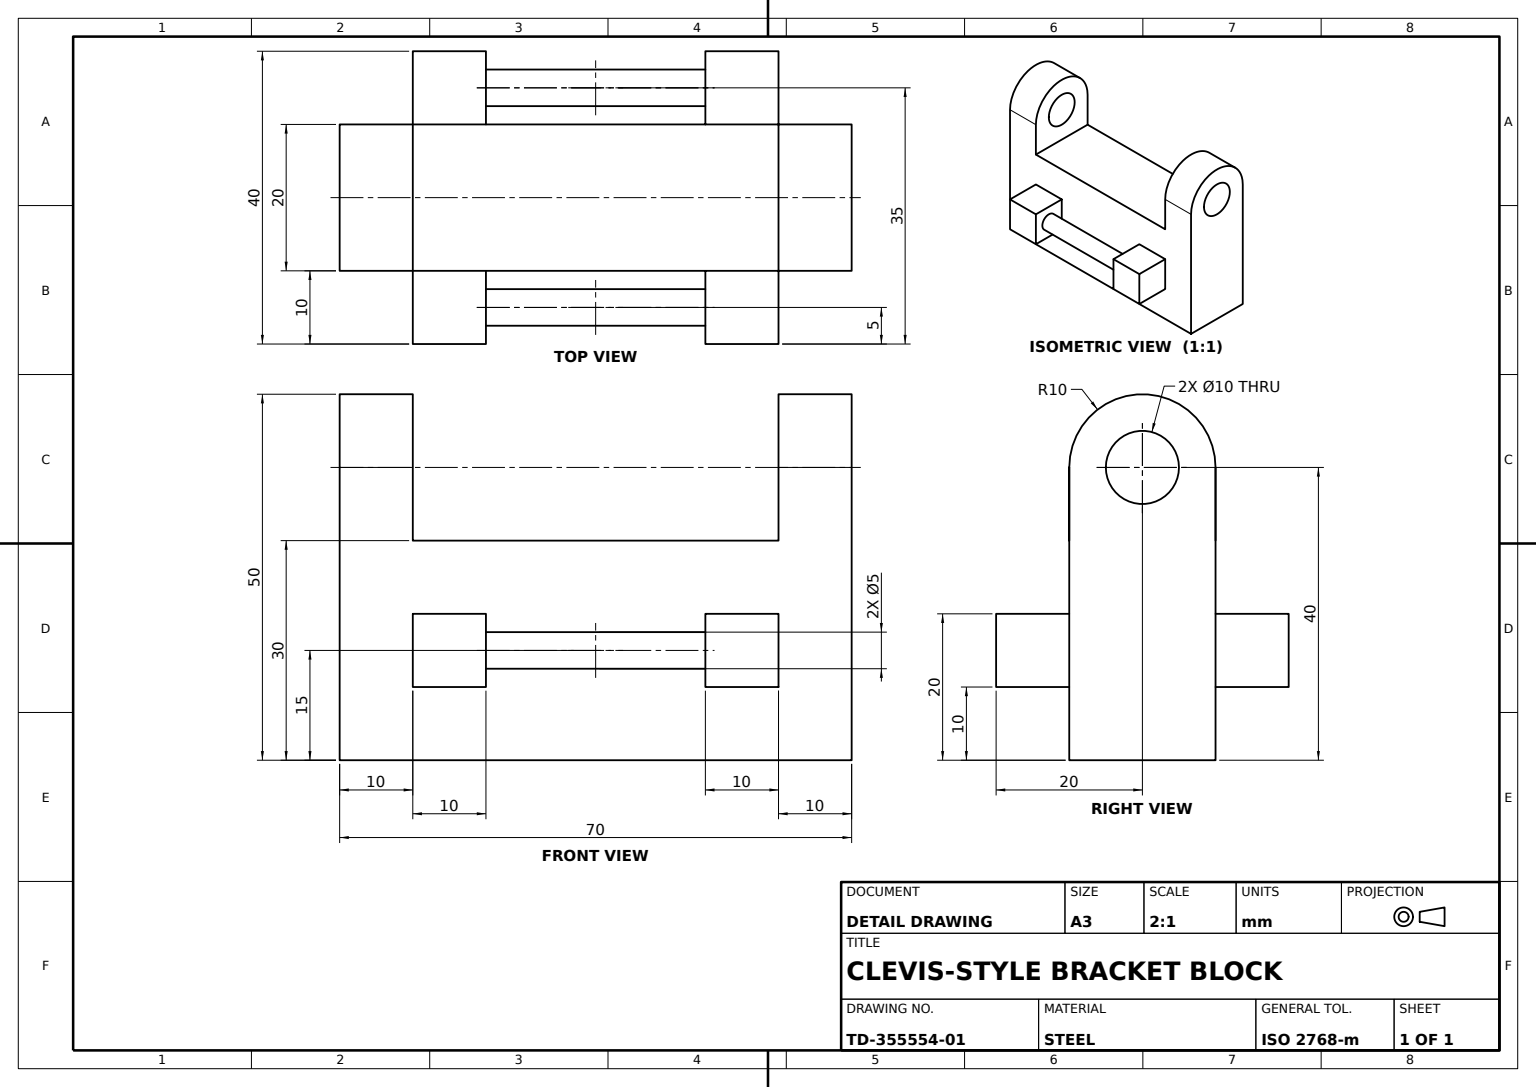
from build123d import *

# Parameters (mm, degrees)
BASE_BLOCK_SKETCH_W   = 70
BASE_BLOCK_SKETCH_H   = 30
BASE_BLOCK_DEPTH      = 20
HINGE_EAR_SKETCH_R    = 5
HINGE_EAR_DEPTH       = 10
SIDE_BLOCK_SKETCH_W   = 10
SIDE_BLOCK_SKETCH_H   = 10
SIDE_BLOCK_DEPTH      = 10
STOP_BLOCK_SKETCH_W   = 10
STOP_BLOCK_SKETCH_H   = 10
STOP_BLOCK_10MM_DEPTH = 10
ROD_SKETCH_R          = 2.5
ROD_30MM_DEPTH        = 30


with BuildPart() as part:
    # Base Block Sketch → Base Block (new body)
    with BuildSketch(Plane.XY):
        with Locations((35, 15)):
            Rectangle(BASE_BLOCK_SKETCH_W, BASE_BLOCK_SKETCH_H)
    extrude(amount=BASE_BLOCK_DEPTH)

    # Hinge Ear Sketch → Hinge Ear (add)
    with BuildSketch(Plane(origin=(0, 0, 0), x_dir=(0, 0, -1), z_dir=(1, 0, 0))):
        with BuildLine():
            Line((-20, 40), (-20, 30))
            Line((-20, 30), (0, 30))
            Line((0, 30), (0, 40))
            ThreePointArc((0, 40), (-10, 50), (-20, 40))
        make_face()
        with Locations((-10, 40)):
            Circle(HINGE_EAR_SKETCH_R, mode=Mode.SUBTRACT)
    hinge_ear = extrude(amount=HINGE_EAR_DEPTH)

    # Hinge Ear Mirror: Hinge Ear across plane
    add(hinge_ear.mirror(Plane(origin=(35, 0, 0), x_dir=(0, 0, 1), z_dir=(1, 0, 0))))

    # Side Block Sketch → Side Block (add)
    with BuildSketch(Plane.XY.offset(20)):
        with Locations((55, 15)):
            Rectangle(SIDE_BLOCK_SKETCH_W, SIDE_BLOCK_SKETCH_H)
    side_block = extrude(amount=SIDE_BLOCK_DEPTH)

    # Stop Block Sketch → Stop Block 10mm (add)
    with BuildSketch(Plane.XY.offset(20)):
        with Locations((15, 15)):
            Rectangle(STOP_BLOCK_SKETCH_W, STOP_BLOCK_SKETCH_H)
    stop_block_10mm = extrude(amount=STOP_BLOCK_10MM_DEPTH)

    # Rod Sketch → Rod 30mm (add)
    with BuildSketch(Plane(origin=(20, 0, 0), x_dir=(0, 0, -1), z_dir=(1, 0, 0))):
        with Locations(Location((-25, 15, 0), (0, 0, 180))):
            Circle(ROD_SKETCH_R)
    rod_30mm = extrude(amount=ROD_30MM_DEPTH)

    # Block and Rod Mirror: Side Block, Stop Block 10mm, Rod 30mm across plane
    add(side_block.mirror(Plane.XY.offset(10)))
    add(stop_block_10mm.mirror(Plane.XY.offset(10)))
    add(rod_30mm.mirror(Plane.XY.offset(10)))


solid = part.part
